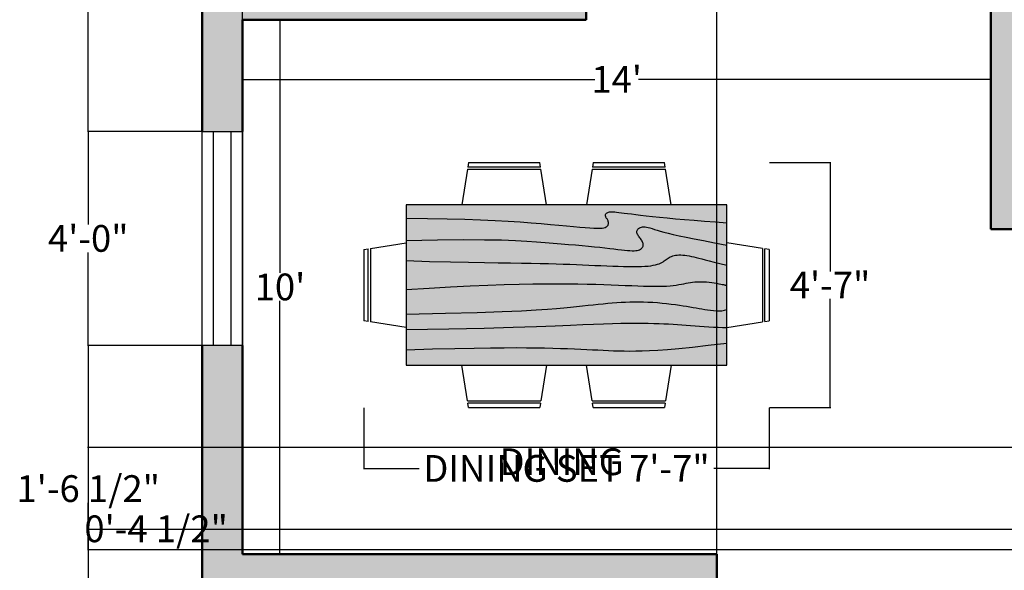
# Model space of a CAD drawing. Units: inches. Extents: x -19 to 426, y -15 to 535.
# Tile 2 of 4: x -19 to 202, y 235 to 359. Entities that reach past the tile are written whole.
import ezdxf

# ---------------------------------------------------------------- set-up
doc = ezdxf.new("R2010")
doc.units = ezdxf.units.IN
doc.header["$MEASUREMENT"] = 0
for name, color, linetype, lineweight in [('A-ANNO-DIMS', 3, 'Continuous', 18), ('A-AREA-IDEN', 7, 'Continuous', 25), ('A-FURN', 40, 'Continuous', 25), ('A-FURN-PATT', 9, 'Continuous', 13), ('A-GLAZ', 40, 'Continuous', 25), ('A-WALL', 7, 'Continuous', 50), ('A-WALL-PATT', 5, 'Continuous', 13)]:
    doc.layers.add(name, color=color, linetype=linetype, lineweight=lineweight)
doc.styles.get("Standard").update_dxf_attribs({"font": 'arial.ttf'})
doc.dimstyles.get("Standard").update_dxf_attribs({"dimtxt": 6, "dimasz": 0.18, "dimexe": 0.18, "dimexo": 0.0625, "dimgap": 0.09, "dimtad": 0, "dimtih": 1, "dimtoh": 1, "dimzin": 0, "dimdsep": 46, "dimlunit": 3, "dimtxsty": 'Standard', "dimcen": 0.09, "dimadec": 0, "dimazin": 0, "dimtfac": 1, "dimtofl": 0, "dimtmove": 0, "dimatfit": 3, "dimfxl": 1, "dimtolj": 1, "dimtzin": 0, "dimarcsym": 0})

# ---------------------------------------------------------------- blocks, each defined once
blk = doc.blocks.new('*D5')
at = {"layer": 'A-ANNO-DIMS', "color": 0, "lineweight": -2, "transparency": 16777216}
for p, q in [((31.49, 359.01), (40.04, 359.01)), ((39.86, 358.83), (39.86, 302.16)), ((39.86, 239.19), (39.86, 295.85)), ((31.49, 239.01), (40.04, 239.01))]:
    blk.add_line(p, q, dxfattribs=at)
at = {"layer": 'A-ANNO-DIMS', "color": 0, "transparency": 16777216}
for points in [[(39.83, 358.83), (39.89, 358.83), (39.86, 359.01)], [(39.83, 239.19), (39.89, 239.19), (39.86, 239.01)]]:
    blk.add_solid(points, dxfattribs=at)
at = {"layer": 'Defpoints', "color": 0, "transparency": 16777216}
for p in [(31.43, 359.01), (31.43, 239.01), (39.86, 239.01)]:
    blk.add_point(p, dxfattribs=at)
at = {"layer": 'A-ANNO-DIMS', "color": 0, "transparency": 16777216, "insert": (39.86, 299.01), "char_height": 6, "attachment_point": 5}
blk.add_mtext("\\A1;10'", dxfattribs=at)
blk = doc.blocks.new('Dining Set - 36 x 72 in.')
for p, q in [((-22, 27.5), (-22.1562, 26.50042)), ((-22, 27.5), (-6, 27.5)), ((-5.8437, 26.49966), (-6, 27.5)), ((6, 27.5), (5.8438, 26.50042)), ((6, 27.5), (22, 27.5)), ((22.1563, 26.49966), (22, 27.5)), ((-22.2343, 26.00059), (-23.4847, 17.99762)), ((-22.2304, 26), (-5.7608, 26)), ((-5.8416, 26.5), (-22.1534, 26.5)), ((-4.5152, 17.99762), (-5.7655, 25.99926)), ((5.7657, 26.00059), (4.5153, 17.99762)), ((5.7696, 26), (22.2392, 26)), ((22.1584, 26.5), (5.8466, 26.5)), ((23.4848, 17.99762), (22.2345, 25.99926)), ((36, 18), (-36, 18)), ((-36, 18), (-36, -18)), ((36, -18), (36, 18)), ((-44.0006, 8.23428), (-35.9976, 9.48474)), ((44.0006, 8.23428), (35.9976, 9.48474)), ((-45.5, 8), (-44.5004, 8.15617)), ((-45.5, 8), (-45.5, -8)), ((-44.5, -8.15843), (-44.5, 8.15338)), ((-44, 8.23041), (-44, -8.23915)), ((44, 8.23041), (44, -8.23915)), ((44.5, -8.15843), (44.5, 8.15338)), ((45.5, 8), (44.5005, 8.15617)), ((45.5, 8), (45.5, -8)), ((-44.4997, -8.15631), (-45.5, -8)), ((-35.9976, -9.48476), (-43.9993, -8.2345)), ((35.9976, -9.48476), (43.9993, -8.2345)), ((44.4997, -8.15631), (45.5, -8)), ((-36, -18), (36, -18)), ((-22.2343, -26.0006), (-23.4847, -17.99762)), ((-4.5152, -17.99762), (-5.7655, -25.99928)), ((5.7657, -26.0006), (4.5153, -17.99762)), ((23.4848, -17.99762), (22.2345, -25.99928)), ((-22.2304, -26), (-5.7608, -26)), ((-22, -27.5), (-22.1562, -26.50044)), ((-5.8416, -26.5), (-22.1534, -26.5)), ((-5.8437, -26.49967), (-6, -27.5)), ((5.7696, -26), (22.2392, -26)), ((6, -27.5), (5.8438, -26.50044)), ((22.1584, -26.5), (5.8466, -26.5)), ((22.1563, -26.49967), (22, -27.5)), ((-22, -27.5), (-6, -27.5)), ((6, -27.5), (22, -27.5))]:
    blk.add_line(p, q)
for points in [[(-36, 15), (-31.1772, 14.97754), (-26.8079, 14.91406), (-22.8538, 14.81543), (-19.276, 14.6875), (-16.0362, 14.53613), (-13.0957, 14.36718), (-10.4159, 14.18652), (-7.9583, 14), (-5.6904, 13.81315), (-3.6035, 13.63021), (-1.6954, 13.45508), (0.0365, 13.29166), (1.5945, 13.14388), (2.9811, 13.01562), (4.1988, 12.9108), (5.25, 12.83333), (6.1393, 12.78613), (6.8802, 12.76823), (7.4883, 12.77767), (7.9792, 12.8125), (8.3685, 12.87077), (8.6719, 12.95052), (8.9049, 13.0498), (9.0833, 13.16666), (9.2205, 13.29899), (9.3216, 13.44401), (9.3895, 13.59879), (9.4271, 13.76041), (9.4373, 13.92594), (9.4232, 14.09245), (9.3875, 14.257), (9.3333, 14.41666), (9.2638, 14.56917), (9.1836, 14.71484), (9.0975, 14.85465), (9.0104, 14.98958), (8.9272, 15.1206), (8.8529, 15.2487), (8.7922, 15.37483), (8.75, 15.5), (8.7305, 15.62467), (8.7344, 15.74739), (8.7617, 15.86621), (8.8125, 15.97916), (8.8867, 16.08431), (8.9844, 16.17968), (9.1055, 16.26334), (9.25, 16.33333), (9.4189, 16.38802), (9.6172, 16.42708), (9.8506, 16.45052), (10.125, 16.45833), (10.4463, 16.45052), (10.8203, 16.42708), (11.2529, 16.38802), (11.75, 16.33333), (12.3184, 16.26318), (12.9694, 16.17838), (13.7151, 16.07991), (14.5677, 15.96875), (15.5395, 15.84586), (16.6426, 15.71224), (17.8893, 15.56884), (19.2917, 15.41666), (20.859, 15.25667), (22.5879, 15.08984), (24.4721, 14.91715), (26.5052, 14.73958), (28.6809, 14.5581), (30.9929, 14.3737), (33.4347, 14.18733), (36, 14)], [(-36, 10), (-28.9766, 10.14274), (-23.1725, 10.20442), (-18.4241, 10.19775), (-14.5677, 10.13541), (-11.4399, 10.03011), (-8.877, 9.89453), (-6.7154, 9.74137), (-4.7917, 9.58333), (-2.9698, 9.43082), (-1.2246, 9.28515), (0.4415, 9.14534), (2.026, 9.01041), (3.5266, 8.87939), (4.9408, 8.7513), (6.266, 8.62516), (7.5, 8.5), (8.6411, 8.37549), (9.6914, 8.2539), (10.6538, 8.13818), (11.5312, 8.03125), (12.3267, 7.93603), (13.043, 7.85547), (13.6831, 7.79248), (14.25, 7.75), (14.7471, 7.7303), (15.1797, 7.73307), (15.5537, 7.75732), (15.875, 7.80208), (16.1494, 7.86637), (16.3828, 7.94922), (16.5811, 8.04964), (16.75, 8.16666), (16.8944, 8.29915), (17.0143, 8.44531), (17.1089, 8.60319), (17.1771, 8.77083), (17.218, 8.94629), (17.2305, 9.1276), (17.2137, 9.31282), (17.1667, 9.5), (17.0895, 9.6875), (16.987, 9.875), (16.8649, 10.0625), (16.7292, 10.25), (16.5856, 10.4375), (16.4401, 10.625), (16.2985, 10.8125), (16.1667, 11), (16.05, 11.18733), (15.9518, 11.3737), (15.8752, 11.5581), (15.8229, 11.73958), (15.798, 11.91715), (15.8034, 12.08984), (15.842, 12.25667), (15.9167, 12.41666), (16.0295, 12.56836), (16.1784, 12.70833), (16.3605, 12.83268), (16.5729, 12.9375), (16.8127, 13.01888), (17.0768, 13.07291), (17.3625, 13.0957), (17.6667, 13.08333), (17.9894, 13.03312), (18.3418, 12.94726), (18.7382, 12.82918), (19.1927, 12.68229), (19.7195, 12.51001), (20.3327, 12.31575), (21.0465, 12.10294), (21.875, 11.875), (22.8357, 11.63354), (23.959, 11.37304), (25.2786, 11.08618), (26.8282, 10.76562), (28.6414, 10.40405), (30.752, 9.99414), (33.1936, 9.52856), (36, 9)], [(-36, 5.5), (-30.7157, 5.3348), (-26.069, 5.20963), (-21.9946, 5.11767), (-18.4271, 5.05208), (-15.3009, 5.00602), (-12.5508, 4.97265), (-10.1112, 4.94515), (-7.9167, 4.91666), (-5.909, 4.88167), (-4.0586, 4.83984), (-2.3429, 4.79215), (-0.7396, 4.73958), (0.7739, 4.6831), (2.22, 4.6237), (3.6213, 4.56233), (5, 4.5), (6.373, 4.43782), (7.7344, 4.3776), (9.0723, 4.32129), (10.375, 4.27083), (11.6309, 4.22819), (12.8281, 4.19531), (13.9551, 4.17415), (15, 4.16666), (15.954, 4.17448), (16.819, 4.19791), (17.6001, 4.23698), (18.3021, 4.29166), (18.9299, 4.36198), (19.4883, 4.44791), (19.9823, 4.54948), (20.4167, 4.66666), (20.7969, 4.79899), (21.1302, 4.94401), (21.4245, 5.09879), (21.6875, 5.26041), (21.9271, 5.42594), (22.1511, 5.59245), (22.3672, 5.757), (22.5834, 5.91666), (22.8065, 6.06868), (23.0404, 6.21093), (23.2879, 6.34147), (23.5521, 6.45833), (23.8358, 6.55957), (24.142, 6.64323), (24.4735, 6.70735), (24.8334, 6.75), (25.2235, 6.76969), (25.642, 6.76692), (26.0858, 6.74267), (26.5521, 6.69791), (27.0379, 6.63362), (27.5404, 6.55078), (28.0565, 6.45036), (28.5834, 6.33333), (29.1242, 6.19987), (29.7071, 6.04687), (30.3661, 5.87044), (31.1354, 5.66666), (32.0493, 5.43164), (33.142, 5.16146), (34.4475, 4.85221), (36, 4.5)], [(-36, -1), (-30.7915, -0.6591), (-26.0195, -0.38216), (-21.6519, -0.16284), (-17.6563, 0.00521), (-14.0005, 0.12833), (-10.6523, 0.21289), (-7.5796, 0.26522), (-4.75, 0.29166), (-2.134, 0.29793), (0.2878, 0.28711), (2.5317, 0.26163), (4.6146, 0.22396), (6.5529, 0.17651), (8.3633, 0.12174), (10.0623, 0.06209), (11.6667, 0), (13.1899, -0.06201), (14.6341, -0.1211), (15.9982, -0.17432), (17.2813, -0.21875), (18.4823, -0.25147), (19.6003, -0.26953), (20.6343, -0.27002), (21.5834, -0.25), (22.4481, -0.20768), (23.2357, -0.14584), (23.9549, -0.06836), (24.6146, 0.02083), (25.2235, 0.11784), (25.7904, 0.21875), (26.3241, 0.31966), (26.8334, 0.41666), (27.3265, 0.50618), (27.8099, 0.58593), (28.2894, 0.65397), (28.7709, 0.70833), (29.2601, 0.74707), (29.763, 0.76823), (30.2855, 0.76985), (30.8334, 0.75), (31.4088, 0.70784), (31.9994, 0.64713), (32.589, 0.57275), (33.1615, 0.48958), (33.7008, 0.4025), (34.1908, 0.3164), (34.6153, 0.23616), (34.9584, 0.16666), (35.2099, 0.11165), (35.3848, 0.07031), (35.504, 0.04069), (35.5886, 0.02083), (35.6594, 0.00879), (35.7377, 0.0026), (35.8442, 0.00032), (36, 0)], [(-36, -6.5), (-27.1843, -6.31267), (-20.084, -6.1263), (-14.469, -5.9419), (-10.1094, -5.76042), (-6.7752, -5.58285), (-4.2363, -5.41016), (-2.2629, -5.24333), (-0.625, -5.08334), (0.8708, -4.93099), (2.2715, -4.78646), (3.5872, -4.64974), (4.8281, -4.52084), (6.0046, -4.39974), (7.127, -4.28646), (8.2053, -4.18099), (9.25, -4.08334), (10.2705, -3.99382), (11.2734, -3.91407), (12.2647, -3.84603), (13.25, -3.79167), (14.2354, -3.75293), (15.2266, -3.73177), (16.2295, -3.73015), (17.25, -3.75), (18.2912, -3.79248), (19.3451, -3.85547), (20.4009, -3.93604), (21.4479, -4.03125), (22.4754, -4.13819), (23.4727, -4.25391), (24.4289, -4.37549), (25.3334, -4.5), (26.1785, -4.62492), (26.9694, -4.74935), (27.7145, -4.87281), (28.4219, -4.99479), (29.1, -5.11483), (29.7572, -5.23242), (30.4016, -5.34709), (31.0417, -5.45834), (31.6837, -5.56437), (32.3262, -5.65821), (32.9658, -5.73153), (33.599, -5.77604), (34.2224, -5.78345), (34.8327, -5.74545), (35.4264, -5.65373), (36, -5.5)], [(-36, -10), (-26.4022, -9.81299), (-18.4675, -9.62891), (-11.9839, -9.45069), (-6.7396, -9.28125), (-2.5226, -9.12354), (0.8789, -8.98047), (3.6769, -8.85498), (6.0833, -8.75), (8.2767, -8.66765), (10.3021, -8.60677), (12.1712, -8.56543), (13.8958, -8.54167), (15.4876, -8.53353), (16.9583, -8.53907), (18.3197, -8.55632), (19.5834, -8.58334), (20.7616, -8.61841), (21.8685, -8.66081), (22.9188, -8.71004), (23.9271, -8.76563), (24.9081, -8.82707), (25.8763, -8.89388), (26.8465, -8.96558), (27.8334, -9.04167), (28.8474, -9.12118), (29.8828, -9.20117), (30.93, -9.27824), (31.9792, -9.34896), (33.0205, -9.40991), (34.0443, -9.45768), (35.0407, -9.48885), (36, -9.5)], [(-36, -14.5), (-30.0881, -14.33513), (-25.0332, -14.21224), (-20.7312, -14.12647), (-17.0781, -14.07292), (-13.97, -14.04671), (-11.3027, -14.04297), (-8.9724, -14.05681), (-6.875, -14.08334), (-4.9224, -14.11833), (-3.0905, -14.16016), (-1.3709, -14.20785), (0.2448, -14.26042), (1.7647, -14.3169), (3.1973, -14.3763), (4.5507, -14.43767), (5.8333, -14.5), (7.0554, -14.5621), (8.235, -14.62175), (9.3922, -14.67652), (10.5469, -14.72396), (11.7192, -14.76164), (12.929, -14.78711), (14.1965, -14.79794), (15.5417, -14.79167), (16.9933, -14.76424), (18.6152, -14.70508), (20.4804, -14.60197), (22.6615, -14.44271), (25.2312, -14.21509), (28.2624, -13.9069), (31.8277, -13.50594), (36, -13)]]:
    blk.add_lwpolyline(points)
blk = doc.blocks.new('*D12')
at = {"layer": 'A-ANNO-DIMS', "color": 0, "lineweight": -2, "transparency": 16777216}
for p, q in [((31.43, 358.94), (31.43, 345.42)), ((199.43, 358.94), (199.43, 345.42)), ((31.61, 345.6), (110.53, 345.6)), ((199.25, 345.6), (120.33, 345.6))]:
    blk.add_line(p, q, dxfattribs=at)
at = {"layer": 'A-ANNO-DIMS', "color": 0, "transparency": 16777216}
for points in [[(31.61, 345.63), (31.61, 345.57), (31.43, 345.6)], [(199.25, 345.63), (199.25, 345.57), (199.43, 345.6)]]:
    blk.add_solid(points, dxfattribs=at)
at = {"layer": 'Defpoints', "color": 0, "transparency": 16777216}
for p in [(31.43, 359.01), (199.43, 359.01), (199.43, 345.6)]:
    blk.add_point(p, dxfattribs=at)
at = {"layer": 'A-ANNO-DIMS', "color": 0, "transparency": 16777216, "insert": (115.43, 345.6), "char_height": 6, "attachment_point": 5}
blk.add_mtext("\\A1;14'", dxfattribs=at)
blk = doc.blocks.new('*D30')
at = {"layer": 'A-ANNO-DIMS', "color": 0, "lineweight": -2, "transparency": 16777216}
for p, q in [((58.67, 271.85), (58.67, 258.08)), ((149.67, 271.85), (149.67, 258.08)), ((58.85, 258.26), (71.11, 258.26)), ((149.49, 258.26), (137.23, 258.26))]:
    blk.add_line(p, q, dxfattribs=at)
at = {"layer": 'A-ANNO-DIMS', "color": 0, "transparency": 16777216}
for points in [[(58.85, 258.29), (58.85, 258.23), (58.67, 258.26)], [(149.49, 258.29), (149.49, 258.23), (149.67, 258.26)]]:
    blk.add_solid(points, dxfattribs=at)
at = {"layer": 'Defpoints', "color": 0, "transparency": 16777216}
for p in [(58.67, 271.91), (149.67, 271.91), (149.67, 258.26)]:
    blk.add_point(p, dxfattribs=at)
at = {"layer": 'A-ANNO-DIMS', "color": 0, "transparency": 16777216, "insert": (104.17, 258.26), "char_height": 6, "attachment_point": 5}
blk.add_mtext('\\A1;DINING SET 7\'-7"', dxfattribs=at)
blk = doc.blocks.new('*D31')
at = {"layer": 'A-ANNO-DIMS', "color": 0, "lineweight": -2, "transparency": 16777216}
for p, q in [((149.73, 326.91), (163.5, 326.91)), ((163.32, 326.73), (163.32, 302.5)), ((163.32, 272.09), (163.32, 296.32)), ((149.73, 271.91), (163.5, 271.91))]:
    blk.add_line(p, q, dxfattribs=at)
at = {"layer": 'A-ANNO-DIMS', "color": 0, "transparency": 16777216}
for points in [[(163.29, 326.73), (163.35, 326.73), (163.32, 326.91)], [(163.29, 272.09), (163.35, 272.09), (163.32, 271.91)]]:
    blk.add_solid(points, dxfattribs=at)
at = {"layer": 'Defpoints', "color": 0, "transparency": 16777216}
for p in [(149.67, 326.91), (163.32, 326.91), (149.67, 271.91)]:
    blk.add_point(p, dxfattribs=at)
at = {"layer": 'A-ANNO-DIMS', "color": 0, "transparency": 16777216, "insert": (163.32, 299.41), "char_height": 6, "attachment_point": 5}
blk.add_mtext('\\A1;4\'-7"', dxfattribs=at)
blk = doc.blocks.new('*D39')
at = {"layer": 'A-ANNO-DIMS', "color": 0, "lineweight": -2, "transparency": 16777216}
for p, q in [((22.37, 285.87), (-3.35, 285.87)), ((-3.17, 285.69), (-3.17, 231.93)), ((-3.17, 171.87), (-3.17, 225.63)), ((22.37, 171.69), (-3.35, 171.69))]:
    blk.add_line(p, q, dxfattribs=at)
at = {"layer": 'A-ANNO-DIMS', "color": 0, "transparency": 16777216}
for points in [[(-3.2, 285.69), (-3.14, 285.69), (-3.17, 285.87)], [(-3.2, 171.87), (-3.14, 171.87), (-3.17, 171.69)]]:
    blk.add_solid(points, dxfattribs=at)
at = {"layer": 'Defpoints', "color": 0, "transparency": 16777216}
for p in [(-3.17, 285.87), (22.43, 285.87), (22.43, 171.69)]:
    blk.add_point(p, dxfattribs=at)
at = {"layer": 'A-ANNO-DIMS', "color": 0, "transparency": 16777216, "insert": (-3.17, 228.78), "char_height": 6, "attachment_point": 5}
blk.add_mtext('\\A1;9\'-6"', dxfattribs=at)
blk = doc.blocks.new('*D40')
at = {"layer": 'A-ANNO-DIMS', "color": 0, "lineweight": -2, "transparency": 16777216}
for p, q in [((22.37, 333.92), (-3.35, 333.92)), ((-3.17, 333.74), (-3.17, 313.05)), ((-3.17, 286.05), (-3.17, 306.74)), ((22.37, 285.87), (-3.35, 285.87))]:
    blk.add_line(p, q, dxfattribs=at)
at = {"layer": 'A-ANNO-DIMS', "color": 0, "transparency": 16777216}
for points in [[(-3.2, 333.74), (-3.14, 333.74), (-3.17, 333.92)], [(-3.2, 286.05), (-3.14, 286.05), (-3.17, 285.87)]]:
    blk.add_solid(points, dxfattribs=at)
at = {"layer": 'Defpoints', "color": 0, "transparency": 16777216}
for p in [(-3.17, 333.92), (22.43, 333.92), (22.43, 285.87)]:
    blk.add_point(p, dxfattribs=at)
at = {"layer": 'A-ANNO-DIMS', "color": 0, "transparency": 16777216, "insert": (-3.17, 309.9), "char_height": 6, "attachment_point": 5}
blk.add_mtext('\\A1;4\'-0"', dxfattribs=at)
blk = doc.blocks.new('*D41')
at = {"layer": 'A-ANNO-DIMS', "color": 0, "lineweight": -2, "transparency": 16777216}
for p, q in [((22.37, 400.98), (-3.35, 400.98)), ((-3.17, 400.8), (-3.17, 370.59)), ((-3.17, 334.1), (-3.17, 364.31)), ((22.37, 333.92), (-3.35, 333.92))]:
    blk.add_line(p, q, dxfattribs=at)
at = {"layer": 'A-ANNO-DIMS', "color": 0, "transparency": 16777216}
for points in [[(-3.2, 400.8), (-3.14, 400.8), (-3.17, 400.98)], [(-3.2, 334.1), (-3.14, 334.1), (-3.17, 333.92)]]:
    blk.add_solid(points, dxfattribs=at)
at = {"layer": 'Defpoints', "color": 0, "transparency": 16777216}
for p in [(-3.17, 400.98), (22.43, 400.98), (22.43, 333.92)]:
    blk.add_point(p, dxfattribs=at)
at = {"layer": 'A-ANNO-DIMS', "color": 0, "transparency": 16777216, "insert": (-3.17, 367.45), "char_height": 6, "attachment_point": 5}
blk.add_mtext('\\A1;5\'-7"', dxfattribs=at)
blk = doc.blocks.new('*D52')
at = {"layer": 'A-ANNO-DIMS', "color": 0, "lineweight": -2, "transparency": 16777216}
for p, q in [((31.43, 239.07), (31.43, 525.79)), ((31.61, 525.61), (67.28, 525.61)), ((137.72, 525.61), (102.06, 525.61)), ((137.9, 239.07), (137.9, 525.79))]:
    blk.add_line(p, q, dxfattribs=at)
at = {"layer": 'A-ANNO-DIMS', "color": 0, "transparency": 16777216}
for points in [[(31.61, 525.64), (31.61, 525.58), (31.43, 525.61)], [(137.72, 525.64), (137.72, 525.58), (137.9, 525.61)]]:
    blk.add_solid(points, dxfattribs=at)
at = {"layer": 'Defpoints', "color": 0, "transparency": 16777216}
for p in [(137.9, 525.61), (31.43, 239.01), (137.9, 239.01)]:
    blk.add_point(p, dxfattribs=at)
at = {"layer": 'A-ANNO-DIMS', "color": 0, "transparency": 16777216, "insert": (84.67, 525.61), "char_height": 6, "attachment_point": 5}
blk.add_mtext('\\A1;8\'-10 1/2"', dxfattribs=at)
blk = doc.blocks.new('*D55')
at = {"layer": 'A-ANNO-DIMS', "color": 0, "lineweight": -2, "transparency": 16777216}
for p, q in [((296.37, 244.52), (-3.35, 244.52)), ((-3.17, 244.52), (-3.17, 244.7)), ((-3.17, 244.7), (-2.99, 244.7)), ((-3.17, 240.19), (-3.17, 244.34)), ((296.37, 240.01), (-3.35, 240.01))]:
    blk.add_line(p, q, dxfattribs=at)
at = {"layer": 'A-ANNO-DIMS', "color": 0, "transparency": 16777216}
for points in [[(-3.2, 244.34), (-3.14, 244.34), (-3.17, 244.52)], [(-3.2, 240.19), (-3.14, 240.19), (-3.17, 240.01)]]:
    blk.add_solid(points, dxfattribs=at)
at = {"layer": 'Defpoints', "color": 0, "transparency": 16777216}
for p in [(-3.17, 244.52), (296.43, 244.52), (296.43, 240.01)]:
    blk.add_point(p, dxfattribs=at)
at = {"layer": 'A-ANNO-DIMS', "color": 0, "transparency": 16777216, "insert": (12.07, 244.7), "char_height": 6, "attachment_point": 5}
blk.add_mtext('\\A1;0\'-4 1/2"', dxfattribs=at)
blk = doc.blocks.new('*D56')
at = {"layer": 'A-ANNO-DIMS', "color": 0, "lineweight": -2, "transparency": 16777216}
for p, q in [((296.37, 262.94), (-3.35, 262.94)), ((-3.17, 262.76), (-3.17, 256.93)), ((-3.17, 244.7), (-3.17, 250.54)), ((296.37, 244.52), (-3.35, 244.52))]:
    blk.add_line(p, q, dxfattribs=at)
at = {"layer": 'A-ANNO-DIMS', "color": 0, "transparency": 16777216}
for points in [[(-3.2, 262.76), (-3.14, 262.76), (-3.17, 262.94)], [(-3.2, 244.7), (-3.14, 244.7), (-3.17, 244.52)]]:
    blk.add_solid(points, dxfattribs=at)
at = {"layer": 'Defpoints', "color": 0, "transparency": 16777216}
for p in [(-3.17, 262.94), (296.43, 262.94), (296.43, 244.52)]:
    blk.add_point(p, dxfattribs=at)
at = {"layer": 'A-ANNO-DIMS', "color": 0, "transparency": 16777216, "insert": (-3.17, 253.73), "char_height": 6, "attachment_point": 5}
blk.add_mtext('\\A1;1\'-6 1/2"', dxfattribs=at)

msp = doc.modelspace()

# ---------------------------------------------------------------- hatches: boundary and pattern name
at = {"layer": 'A-FURN-PATT'}
h = msp.add_hatch(color=256, dxfattribs=at)
h.dxf.hatch_style = 1
h.paths.add_polyline_path([(112.909, 315.288), (113.096, 315.552), (113.34, 315.72), (113.675, 315.829), (114.021, 315.864), (114.296, 315.872), (114.617, 315.864), (114.991, 315.84), (115.424, 315.801), (115.921, 315.747), (116.489, 315.677), (117.14, 315.592), (117.886, 315.493), (118.738, 315.382), (119.71, 315.259), (120.813, 315.126), (122.06, 314.982), (123.462, 314.83), (125.03, 314.67), (126.759, 314.503), (128.643, 314.331), (130.676, 314.153), (132.852, 313.971), (135.164, 313.787), (137.605, 313.601), (140.171, 313.413), (140.171, 317.413), (68.171, 317.413), (68.171, 314.413), (72.994, 314.391), (77.363, 314.327), (81.317, 314.229), (84.895, 314.101), (88.135, 313.949), (91.075, 313.781), (93.755, 313.6), (96.212, 313.413), (98.48, 313.227), (100.567, 313.044), (102.475, 312.868), (104.207, 312.705), (105.765, 312.557), (107.152, 312.429), (108.37, 312.324), (109.421, 312.247), (110.31, 312.199), (111.051, 312.182), (111.659, 312.191), (112.15, 312.226), (112.539, 312.284), (112.843, 312.364), (113.076, 312.463), (113.254, 312.58), (113.391, 312.712), (113.492, 312.857), (113.56, 313.012), (113.598, 313.174), (113.608, 313.339), (113.594, 313.506), (113.558, 313.67), (113.504, 313.83), (113.435, 313.983), (113.354, 314.128), (113.268, 314.268), (113.052, 314.603), (112.898, 314.924)])
h.paths.add_polyline_path([(121.248, 312.486), (121.533, 312.509), (121.837, 312.497), (122.16, 312.446), (122.513, 312.361), (122.909, 312.243), (123.363, 312.096), (123.89, 311.923), (124.503, 311.729), (125.217, 311.516), (126.046, 311.288), (127.006, 311.047), (128.13, 310.786), (129.449, 310.5), (130.999, 310.179), (132.812, 309.817), (134.923, 309.407), (137.364, 308.942), (140.171, 308.413), (140.171, 313.413), (137.605, 313.601), (135.164, 313.787), (132.852, 313.971), (130.676, 314.153), (128.643, 314.331), (126.759, 314.503), (125.03, 314.67), (123.462, 314.83), (122.06, 314.982), (120.813, 315.126), (119.71, 315.259), (118.738, 315.382), (117.886, 315.493), (117.14, 315.592), (116.489, 315.677), (115.921, 315.747), (115.424, 315.801), (114.991, 315.84), (114.617, 315.864), (114.296, 315.872), (114.021, 315.864), (113.788, 315.84), (113.59, 315.801), (113.421, 315.747), (113.276, 315.677), (113.155, 315.593), (113.057, 315.498), (112.983, 315.393), (112.932, 315.28), (112.905, 315.161), (112.901, 315.038), (112.921, 314.913), (112.963, 314.788), (113.024, 314.662), (113.098, 314.534), (113.181, 314.403), (113.391, 314.077), (113.541, 313.748), (113.613, 313.418), (113.592, 313.085), (113.456, 312.775), (113.178, 312.507), (112.843, 312.364), (112.539, 312.284), (112.15, 312.226), (111.659, 312.191), (111.051, 312.182), (110.31, 312.199), (109.421, 312.247), (108.37, 312.324), (107.152, 312.429), (105.765, 312.557), (104.207, 312.705), (102.475, 312.868), (100.567, 313.044), (98.48, 313.227), (96.212, 313.413), (93.755, 313.6), (91.075, 313.781), (88.135, 313.949), (84.895, 314.101), (81.317, 314.229), (77.363, 314.327), (72.994, 314.391), (68.171, 314.413), (68.171, 309.413), (75.194, 309.556), (80.998, 309.618), (85.747, 309.611), (89.603, 309.549), (92.731, 309.443), (95.294, 309.308), (97.455, 309.155), (99.379, 308.997), (101.201, 308.844), (102.946, 308.699), (104.612, 308.559), (106.197, 308.424), (107.697, 308.293), (109.112, 308.165), (110.437, 308.039), (111.671, 307.913), (112.812, 307.789), (113.862, 307.667), (114.825, 307.552), (115.702, 307.445), (116.497, 307.349), (117.214, 307.269), (117.854, 307.206), (118.421, 307.163), (118.918, 307.144), (119.35, 307.146), (119.724, 307.171), (120.046, 307.215), (120.32, 307.28), (120.554, 307.363), (120.752, 307.463), (120.921, 307.58), (121.065, 307.713), (121.185, 307.859), (121.28, 308.017), (121.348, 308.184), (121.389, 308.36), (121.401, 308.541), (121.384, 308.726), (121.337, 308.913), (121.26, 309.101), (121.158, 309.288), (121.036, 309.476), (120.9, 309.663), (120.756, 309.851), (120.507, 310.172), (120.266, 310.516), (120.071, 310.885), (119.966, 311.248), (119.977, 311.593), (120.125, 311.911), (120.426, 312.194), (120.856, 312.406)])
h.paths.add_polyline_path([(140.171, 308.413), (137.364, 308.942), (134.923, 309.407), (132.812, 309.817), (130.999, 310.179), (129.449, 310.5), (128.13, 310.786), (127.006, 311.047), (126.046, 311.288), (125.217, 311.516), (124.503, 311.729), (123.89, 311.923), (123.363, 312.096), (122.909, 312.243), (122.513, 312.361), (122.16, 312.446), (121.837, 312.497), (121.533, 312.509), (121.248, 312.486), (120.983, 312.432), (120.744, 312.351), (120.531, 312.246), (120.349, 312.122), (120.2, 311.982), (120.087, 311.83), (120.013, 311.67), (119.974, 311.503), (119.969, 311.331), (119.994, 311.153), (120.046, 310.971), (120.123, 310.787), (120.221, 310.601), (120.337, 310.413), (120.469, 310.226), (120.611, 310.038), (120.874, 309.7), (121.116, 309.365), (121.316, 308.999), (121.408, 308.634), (121.383, 308.269), (121.245, 307.932), (121.004, 307.637), (120.663, 307.401), (120.32, 307.28), (120.046, 307.215), (119.724, 307.171), (119.35, 307.146), (118.918, 307.144), (118.421, 307.163), (117.854, 307.206), (117.214, 307.269), (116.497, 307.349), (115.702, 307.445), (114.825, 307.552), (113.862, 307.667), (112.812, 307.789), (111.671, 307.913), (110.437, 308.039), (109.112, 308.165), (107.697, 308.293), (106.197, 308.424), (104.612, 308.559), (102.946, 308.699), (101.201, 308.844), (99.379, 308.997), (97.455, 309.155), (95.294, 309.308), (92.731, 309.443), (89.603, 309.549), (85.747, 309.611), (80.998, 309.618), (75.194, 309.556), (68.171, 309.413), (68.171, 304.913), (73.455, 304.748), (78.102, 304.623), (82.176, 304.531), (85.744, 304.465), (88.87, 304.419), (91.62, 304.386), (94.06, 304.359), (96.254, 304.33), (98.262, 304.295), (100.112, 304.253), (101.828, 304.206), (103.431, 304.153), (104.945, 304.096), (106.391, 304.037), (107.792, 303.976), (109.171, 303.913), (110.544, 303.851), (111.905, 303.791), (113.243, 303.735), (114.546, 303.684), (115.802, 303.642), (116.999, 303.609), (118.126, 303.588), (119.171, 303.58), (120.125, 303.588), (120.99, 303.611), (121.771, 303.65), (122.473, 303.705), (123.101, 303.775), (123.659, 303.861), (124.153, 303.963), (124.587, 304.08), (124.968, 304.212), (125.301, 304.357), (125.595, 304.512), (125.858, 304.674), (126.098, 304.839), (126.322, 305.006), (126.692, 305.288), (127.1, 305.566), (127.459, 305.755), (127.723, 305.872), (128.007, 305.973), (128.313, 306.057), (128.644, 306.121), (129.004, 306.163), (129.394, 306.183), (129.813, 306.18), (130.257, 306.156), (130.723, 306.111), (131.209, 306.047), (131.711, 305.964), (132.227, 305.864), (132.754, 305.747), (133.295, 305.613), (133.878, 305.46), (134.537, 305.284), (135.306, 305.08), (136.22, 304.845), (137.313, 304.575), (138.618, 304.266), (140.171, 303.913)])
h.paths.add_polyline_path([(140.171, 303.913), (138.618, 304.266), (137.313, 304.575), (136.22, 304.845), (135.306, 305.08), (134.537, 305.284), (133.878, 305.46), (133.295, 305.613), (132.754, 305.747), (132.227, 305.864), (131.711, 305.964), (131.209, 306.047), (130.723, 306.111), (130.257, 306.156), (129.813, 306.18), (129.394, 306.183), (129.004, 306.163), (128.644, 306.121), (128.313, 306.057), (128.007, 305.973), (127.723, 305.872), (127.459, 305.755), (127.211, 305.624), (126.977, 305.482), (126.754, 305.33), (126.538, 305.17), (126.155, 304.879), (125.858, 304.674), (125.595, 304.512), (125.301, 304.357), (124.968, 304.212), (124.587, 304.08), (124.153, 303.963), (123.659, 303.861), (123.101, 303.775), (122.473, 303.705), (121.771, 303.65), (120.99, 303.611), (120.125, 303.588), (119.171, 303.58), (118.126, 303.588), (116.999, 303.609), (115.802, 303.642), (114.546, 303.684), (113.243, 303.735), (111.905, 303.791), (110.544, 303.851), (109.171, 303.913), (107.792, 303.976), (106.391, 304.037), (104.945, 304.096), (103.431, 304.153), (101.828, 304.206), (100.112, 304.253), (98.262, 304.295), (96.254, 304.33), (94.06, 304.359), (91.62, 304.386), (88.87, 304.419), (85.744, 304.465), (82.176, 304.531), (78.102, 304.623), (73.455, 304.748), (68.171, 304.913), (68.171, 298.413), (73.379, 298.754), (78.151, 299.031), (82.519, 299.251), (86.514, 299.419), (90.17, 299.542), (93.518, 299.626), (96.591, 299.679), (99.421, 299.705), (102.037, 299.711), (104.459, 299.7), (106.702, 299.675), (108.785, 299.637), (110.724, 299.59), (112.534, 299.535), (114.233, 299.475), (115.837, 299.413), (117.361, 299.351), (118.805, 299.292), (120.169, 299.239), (121.452, 299.195), (122.653, 299.162), (123.771, 299.144), (124.805, 299.143), (125.754, 299.163), (126.619, 299.206), (127.406, 299.268), (128.126, 299.345), (128.785, 299.434), (129.394, 299.531), (129.961, 299.632), (130.495, 299.733), (131.004, 299.83), (131.497, 299.92), (131.981, 299.999), (132.46, 300.067), (132.942, 300.122), (133.431, 300.16), (133.934, 300.182), (134.456, 300.183), (135.004, 300.163), (135.58, 300.121), (136.17, 300.06), (136.76, 299.986), (137.332, 299.903), (137.872, 299.816), (138.362, 299.73), (138.786, 299.65), (139.26, 299.553), (139.779, 299.431), (139.83, 299.422), (139.908, 299.416), (140.015, 299.414), (140.171, 299.413)])
h.paths.add_polyline_path([(140.171, 299.413), (139.845, 299.414), (139.675, 299.454), (139.556, 299.484), (139.381, 299.525), (139.129, 299.58), (138.786, 299.65), (138.362, 299.73), (137.872, 299.816), (137.332, 299.903), (136.76, 299.986), (136.17, 300.06), (135.58, 300.121), (135.004, 300.163), (134.456, 300.183), (133.934, 300.182), (133.431, 300.16), (132.942, 300.122), (132.46, 300.067), (131.981, 299.999), (131.497, 299.92), (131.004, 299.83), (130.495, 299.733), (129.961, 299.632), (129.394, 299.531), (128.785, 299.434), (128.126, 299.345), (127.406, 299.268), (126.619, 299.206), (125.754, 299.163), (124.805, 299.143), (123.771, 299.144), (122.653, 299.162), (121.452, 299.195), (120.169, 299.239), (118.805, 299.292), (117.361, 299.351), (115.837, 299.413), (114.233, 299.475), (112.534, 299.535), (110.724, 299.59), (108.785, 299.637), (106.702, 299.675), (104.459, 299.7), (102.037, 299.711), (99.421, 299.705), (96.591, 299.679), (93.518, 299.626), (90.17, 299.542), (86.514, 299.419), (82.519, 299.251), (78.151, 299.031), (73.379, 298.754), (68.171, 298.413), (68.171, 292.913), (76.986, 293.101), (84.087, 293.287), (89.702, 293.471), (94.061, 293.653), (97.396, 293.831), (99.934, 294.003), (101.908, 294.17), (103.546, 294.33), (105.042, 294.482), (106.442, 294.627), (107.758, 294.764), (108.999, 294.893), (110.175, 295.014), (111.298, 295.127), (112.376, 295.232), (113.421, 295.33), (114.441, 295.42), (115.444, 295.499), (116.435, 295.567), (117.421, 295.622), (118.406, 295.66), (119.397, 295.682), (120.4, 295.683), (121.421, 295.663), (122.462, 295.621), (123.516, 295.558), (124.572, 295.477), (125.619, 295.382), (126.646, 295.275), (127.643, 295.159), (128.6, 295.038), (129.504, 294.913), (130.349, 294.788), (131.14, 294.664), (131.885, 294.541), (132.593, 294.419), (133.271, 294.299), (133.928, 294.181), (134.572, 294.066), (135.212, 293.955), (135.854, 293.849), (136.497, 293.755), (137.137, 293.682), (137.77, 293.637), (138.393, 293.63), (139.003, 293.668), (139.597, 293.76), (140.171, 293.913)])
h.paths.add_polyline_path([(140.171, 293.913), (139.597, 293.76), (139.003, 293.668), (138.393, 293.63), (137.77, 293.637), (137.137, 293.682), (136.497, 293.755), (135.854, 293.849), (135.212, 293.955), (134.572, 294.066), (133.928, 294.181), (133.271, 294.299), (132.593, 294.419), (131.885, 294.541), (131.14, 294.664), (130.349, 294.788), (129.504, 294.913), (128.6, 295.038), (127.643, 295.159), (126.646, 295.275), (125.619, 295.382), (124.572, 295.477), (123.516, 295.558), (122.462, 295.621), (121.421, 295.663), (120.4, 295.683), (119.397, 295.682), (118.406, 295.66), (117.421, 295.622), (116.435, 295.567), (115.444, 295.499), (114.441, 295.42), (113.421, 295.33), (112.376, 295.232), (111.298, 295.127), (110.175, 295.014), (108.999, 294.893), (107.758, 294.764), (106.442, 294.627), (105.042, 294.482), (103.546, 294.33), (101.908, 294.17), (99.934, 294.003), (97.396, 293.831), (94.061, 293.653), (89.702, 293.471), (84.087, 293.287), (76.986, 293.101), (68.171, 292.913), (68.171, 289.413), (77.769, 289.6), (85.703, 289.784), (92.187, 289.963), (97.431, 290.132), (101.648, 290.29), (105.05, 290.433), (107.848, 290.558), (110.254, 290.663), (112.447, 290.746), (114.473, 290.807), (116.342, 290.848), (118.067, 290.872), (119.658, 290.88), (121.129, 290.874), (122.49, 290.857), (123.754, 290.83), (124.932, 290.795), (126.039, 290.753), (127.09, 290.703), (128.098, 290.648), (129.079, 290.586), (130.047, 290.519), (131.017, 290.448), (132.004, 290.372), (133.018, 290.292), (134.054, 290.212), (135.101, 290.135), (136.15, 290.064), (137.191, 290.003), (138.215, 289.956), (139.211, 289.925), (140.078, 289.914), (140.171, 289.929)])
h.paths.add_polyline_path([(140.171, 286.413), (140.171, 289.913), (139.211, 289.925), (138.215, 289.956), (137.191, 290.003), (136.15, 290.064), (135.101, 290.135), (134.054, 290.212), (133.018, 290.292), (132.004, 290.372), (131.017, 290.448), (130.047, 290.519), (129.079, 290.586), (128.098, 290.648), (127.09, 290.703), (126.039, 290.753), (124.932, 290.795), (123.754, 290.83), (122.49, 290.857), (121.129, 290.874), (119.658, 290.88), (118.067, 290.872), (116.342, 290.848), (114.473, 290.807), (112.447, 290.746), (110.254, 290.663), (107.848, 290.558), (105.05, 290.433), (101.648, 290.29), (97.431, 290.132), (92.187, 289.963), (85.703, 289.784), (77.769, 289.6), (68.171, 289.413), (68.171, 284.913), (74.083, 285.078), (79.138, 285.201), (83.44, 285.287), (87.093, 285.34), (90.201, 285.367), (92.868, 285.37), (95.198, 285.357), (97.296, 285.33), (99.248, 285.295), (101.08, 285.253), (102.8, 285.206), (104.416, 285.153), (105.935, 285.096), (107.368, 285.037), (108.721, 284.976), (110.004, 284.913), (111.226, 284.851), (112.406, 284.792), (113.563, 284.737), (114.718, 284.689), (115.89, 284.652), (117.1, 284.626), (118.367, 284.615), (119.712, 284.622), (121.164, 284.649), (122.786, 284.708), (124.651, 284.811), (126.832, 284.971), (129.402, 285.198), (132.433, 285.506), (135.998, 285.907)])
h.paths.add_polyline_path([(140.171, 286.413), (135.998, 285.907), (132.433, 285.506), (129.402, 285.198), (126.832, 284.971), (124.651, 284.811), (122.786, 284.708), (121.164, 284.649), (119.712, 284.622), (118.367, 284.615), (117.1, 284.626), (115.89, 284.652), (114.718, 284.689), (113.563, 284.737), (112.406, 284.792), (111.226, 284.851), (110.004, 284.913), (108.721, 284.976), (107.368, 285.037), (105.935, 285.096), (104.416, 285.153), (102.8, 285.206), (101.08, 285.253), (99.248, 285.295), (97.296, 285.33), (95.198, 285.357), (92.868, 285.37), (90.201, 285.367), (87.093, 285.34), (83.44, 285.287), (79.138, 285.201), (74.083, 285.078), (68.171, 284.913), (68.171, 281.413), (140.171, 281.413)])
at = {"layer": 'A-WALL-PATT'}
h = msp.add_hatch(color=256, dxfattribs=at)
h.dxf.hatch_style = 1
h.paths.add_polyline_path([(205.432, 491.007), (254.275, 491.007), (254.275, 500.007), (22.432, 500.007), (22.432, 449.048), (31.432, 449.048), (31.432, 491.007), (199.432, 491.007), (199.432, 312.007), (225.033, 312.007), (225.033, 315.882), (225.033, 317.007), (205.432, 317.007)])
h.paths.add_polyline_path([(382.432, 500.007), (314.275, 500.007), (314.275, 491.007), (373.432, 491.007), (373.432, 423.411), (382.432, 423.411)])
h.paths.add_polyline_path([(382.432, 363.411), (373.432, 363.411), (373.432, 317.007), (250.847, 317.007, -0.0108825), (250.871, 315.882), (250.871, 312.007), (296.432, 312.007), (296.432, 262.945), (299.196, 262.945, -0.0304399), (301.432, 262.809), (301.432, 312.007), (373.432, 312.007), (373.432, 284.151), (382.432, 284.151)])
h = msp.add_hatch(color=256, dxfattribs=at)
h.dxf.hatch_style = 1
h.paths.add_polyline_path([(108.594, 365.007), (31.432, 365.007), (31.432, 400.979), (22.432, 400.979), (22.432, 333.921), (31.432, 333.921), (31.432, 359.007), (108.594, 359.007)])
h = msp.add_hatch(color=256, dxfattribs=at)
h.dxf.hatch_style = 1
h.paths.add_polyline_path([(31.432, 233.007), (130.834, 233.007), (137.904, 233.007), (137.904, 239.007), (31.432, 239.007), (31.432, 285.874), (22.432, 285.874), (22.432, 171.689), (31.432, 171.689)])
h.paths.add_polyline_path([(31.432, 111.689), (22.432, 111.689), (22.432, 20.007), (46.182, 20.007), (46.182, 26.007), (46.182, 29.007), (31.432, 29.007)])
h.paths.add_polyline_path([(134.169, 29.007), (86.07, 29.007, -0.0187698), (86.182, 26.007), (86.182, 20.007), (134.169, 20.007)])
h.paths.add_polyline_path([(382.432, 50.634), (373.432, 50.634), (373.432, 29.007), (194.169, 29.007), (194.169, 20.007), (382.432, 20.007)])
h.paths.add_polyline_path([(382.432, 148.923), (373.432, 148.923), (373.432, 115.007), (253.432, 115.007), (253.432, 122.516), (253.083, 122.516), (248.432, 122.516), (248.432, 115.007), (238.432, 115.007), (238.432, 110.007), (373.432, 110.007), (373.432, 98.634), (382.432, 98.634)])

# ---------------------------------------------------------------- linework, layer by layer
at = {"layer": 'A-GLAZ'}
for p, q in [((24.932, 285.874), (24.932, 333.921)), ((28.932, 285.874), (28.932, 333.921))]:
    msp.add_line(p, q, dxfattribs=at)
msp.add_lwpolyline([(22.432, 333.921), (31.432, 333.921), (31.432, 285.874), (22.432, 285.874)], close=True, dxfattribs=at)
at = {"layer": 'A-WALL'}
for p, q in [((108.594, 365.007), (108.594, 359.007)), ((137.904, 239.007), (137.904, 233.007))]:
    msp.add_line(p, q, dxfattribs=at)
for points in [[(199.432, 491.007), (199.432, 312.007)], [(22.432, 400.979), (22.432, 333.874)], [(31.432, 359.007), (31.432, 333.874)], [(108.594, 359.007), (31.432, 359.007)], [(199.432, 359.007), (199.432, 312.007)], [(296.432, 312.007), (199.432, 312.007)], [(22.432, 285.874), (22.432, 171.689)], [(31.432, 285.874), (31.432, 239.007)], [(31.432, 239.007), (137.904, 239.007)]]:
    msp.add_lwpolyline(points, dxfattribs=at)

# ---------------------------------------------------------------- block references
at = {"layer": 'A-FURN'}
msp.add_blockref('Dining Set - 36 x 72 in.', (104.171, 299.413), dxfattribs=at)

# ---------------------------------------------------------------- texts
at = {"layer": 'A-AREA-IDEN', "insert": (89.137, 262.761), "char_height": 6, "attachment_point": 1}
msp.add_mtext_dynamic_manual_height_columns('{DINING}', width=105.43776, gutter_width=1, heights=[0.207], dxfattribs=at)

# ---------------------------------------------------------------- dimensions: what is measured, and where the dimension line sits
at = {"layer": 'A-ANNO-DIMS'}
for base, p1, p2, override, picture, middle in [((137.904, 525.607), (31.432, 239.007), (137.904, 239.007), {"dimdec": 1, "dimlfac": 1, "dimrnd": 0, "dimzin": 1, "dimdsep": 46, "dimlunit": 4, "dimfrac": 2}, '*D52', (84.668, 525.607)), ((199.432, 345.596), (31.432, 359.007), (199.432, 359.007), {"dimclrd": 0, "dimclre": 0, "dimclrt": 0}, '*D12', (115.432, 345.596))]:
    dim = msp.add_linear_dim(base=base, p1=p1, p2=p2, dimstyle='Standard', override=override, dxfattribs=at)
    dim.commit()
    dim.dimension.update_dxf_attribs({"geometry": picture, "text_midpoint": middle})
for base, p1, p2, override, picture, middle in [((-3.168, 400.979), (22.432, 333.921), (22.432, 400.979), {"dimdec": 1, "dimlfac": 1, "dimrnd": 0, "dimzin": 1, "dimdsep": 46, "dimlunit": 4, "dimfrac": 2}, '*D41', (-3.168, 367.45)), ((39.856, 239.007), (31.432, 359.007), (31.432, 239.007), {"dimclrd": 0, "dimclre": 0, "dimclrt": 0}, '*D5', (39.856, 299.007)), ((-3.168, 333.921), (22.432, 285.874), (22.432, 333.921), {"dimdec": 1, "dimlfac": 1, "dimrnd": 0, "dimzin": 1, "dimdsep": 46, "dimlunit": 4, "dimfrac": 2}, '*D40', (-3.168, 309.898)), ((163.321, 326.913), (149.671, 271.913), (149.671, 326.913), {"dimdec": 1, "dimlfac": 1, "dimrnd": 0, "dimzin": 1, "dimdsep": 46, "dimlunit": 4, "dimfrac": 2}, '*D31', (163.321, 299.413)), ((-3.168, 285.874), (22.432, 171.689), (22.432, 285.874), {"dimdec": 1, "dimlfac": 1, "dimrnd": 0, "dimzin": 1, "dimdsep": 46, "dimlunit": 4, "dimfrac": 2}, '*D39', (-3.168, 228.781)), ((-3.168, 262.945), (296.432, 244.523), (296.432, 262.945), {"dimdec": 1, "dimlfac": 1, "dimrnd": 0, "dimzin": 1, "dimdsep": 46, "dimlunit": 4, "dimfrac": 2}, '*D56', (-3.168, 253.734)), ((-3.168, 244.523), (296.432, 240.007), (296.432, 244.523), {"dimdec": 1, "dimlfac": 1, "dimrnd": 0, "dimzin": 1, "dimdsep": 46, "dimlunit": 4, "dimfrac": 2}, '*D55', (12.068, 244.703))]:
    dim = msp.add_linear_dim(base=base, p1=p1, p2=p2, angle=90, dimstyle='Standard', override=override, dxfattribs=at)
    dim.commit()
    dim.dimension.update_dxf_attribs({"geometry": picture, "text_midpoint": middle})
dim = msp.add_linear_dim(base=(149.671, 258.263), p1=(58.671, 271.913), p2=(149.671, 271.913), text='DINING SET <>', dimstyle='Standard', override={"dimdec": 1, "dimlfac": 1, "dimrnd": 0, "dimzin": 1, "dimdsep": 46, "dimlunit": 4, "dimfrac": 2}, dxfattribs=at)
dim.commit()
dim.dimension.update_dxf_attribs({"geometry": '*D30', "text_midpoint": (104.171, 258.263)})

doc.saveas('drawing.dxf')
